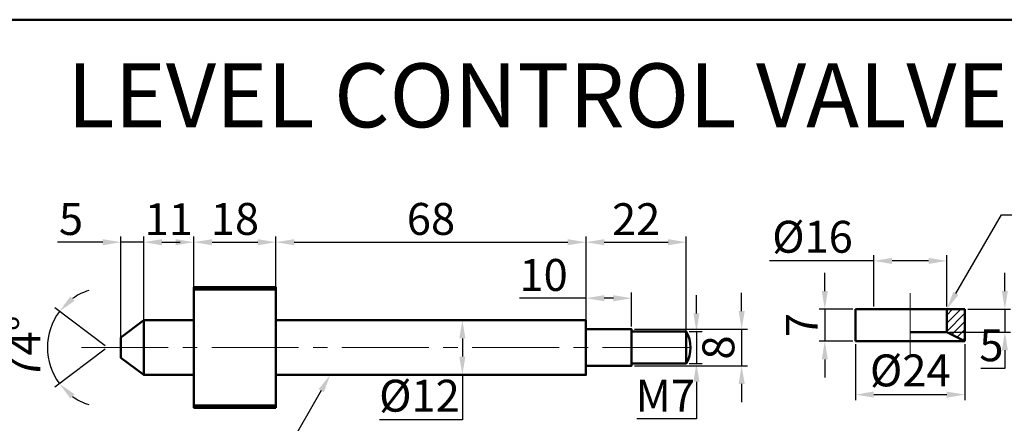
# Model space of a CAD drawing. Units: millimetres. Extents: x 123 to 731, y 468 to 864.
# Tile 4 of 5: x 328 to 544, y 775 to 864. Entities that reach past the tile are written whole.
import ezdxf
from ezdxf import colors
from ezdxf.entities.mleader import LeaderData, LeaderLine
from ezdxf.math import Vec2, Vec3

# ---------------------------------------------------------------- set-up
doc = ezdxf.new("R2010")
doc.units = ezdxf.units.MM
doc.linetypes.add('CENTER2', pattern=[28.575, 19.05, -3.175, 3.175, -3.175])
for name, color, linetype, lineweight in [('M-CNTR', 1, 'CENTER2', 18), ('M-DIMS', 2, 'Continuous', 25), ('M-HATC', 8, 'Continuous', 18), ('M-OUTL', 7, 'Continuous', 50), ('M-TEXT', 3, 'Continuous', 25)]:
    doc.layers.add(name, color=color, linetype=linetype, lineweight=lineweight)
doc.styles.get("Standard").update_dxf_attribs({"font": 'arial.ttf'})
doc.dimstyles.new('ISO-25', dxfattribs={"dimtxt": 7, "dimasz": 4, "dimexe": 1.25, "dimexo": 0.625, "dimtad": 1, "dimtoh": 1, "dimtxsty": 'Standard', "dimcen": 2.5, "dimadec": 0, "dimazin": 0, "dimtfac": 1, "dimtmove": 0, "dimatfit": 3, "dimfxl": 1, "dimarcsym": 0})

# ---------------------------------------------------------------- blocks, each defined once
blk = doc.blocks.new('*U27')
at = {"layer": 'M-CNTR', "color": 0, "transparency": 16777216}
blk.add_line((-76.67, 0), (58.73, 0), dxfattribs=at)
blk = doc.blocks.new('*D28')
at = {"layer": 'Defpoints', "color": 0, "transparency": 16777216}
for p in [(355.16, 798.03), (334.32, 794.85), (350.16, 794.26), (350.16, 789.8), (355.16, 786.03)]:
    blk.add_point(p, dxfattribs=at)
at = {"layer": 'M-DIMS', "color": 0, "lineweight": -2, "transparency": 16777216}
for p, q in [((346.7, 792.41), (335.67, 800.72)), ((346.7, 791.65), (335.67, 783.34))]:
    blk.add_line(p, q, dxfattribs=at)
for start, end in [(108.0972, 125.5486), (143, 217), (234.4514, 251.9028)]:
    blk.add_arc((347.2, 792.03), 13.18, start, end, dxfattribs=at)
at = {"layer": 'M-DIMS', "color": 0, "transparency": 16777216}
for points in [[(340, 802.28), (339.07, 803.23), (336.67, 799.97)], [(339.07, 780.83), (340, 781.78), (336.67, 784.1)]]:
    blk.add_solid(points, dxfattribs=at)
at = {"layer": 'M-DIMS', "color": 0, "transparency": 16777216, "insert": (329.89, 792.03), "char_height": 7, "attachment_point": 5, "rotation": 90}
blk.add_mtext('74°', dxfattribs=at)
blk = doc.blocks.new('*D29')
at = {"layer": 'Defpoints', "color": 0, "transparency": 16777216}
for p in [(355.16, 815.14), (350.16, 792.03), (355.16, 792.03)]:
    blk.add_point(p, dxfattribs=at)
at = {"layer": 'M-DIMS', "color": 0, "lineweight": -2, "transparency": 16777216}
for p, q in [((350.16, 792.66), (350.16, 816.39)), ((355.16, 792.66), (355.16, 816.39)), ((346.16, 815.14), (336.27, 815.14)), ((355.16, 815.14), (350.16, 815.14)), ((359.16, 815.14), (363.16, 815.14))]:
    blk.add_line(p, q, dxfattribs=at)
at = {"layer": 'M-DIMS', "color": 0, "transparency": 16777216}
for points in [[(346.16, 815.8), (346.16, 814.47), (350.16, 815.14)], [(359.16, 815.8), (359.16, 814.47), (355.16, 815.14)]]:
    blk.add_solid(points, dxfattribs=at)
at = {"layer": 'M-DIMS', "color": 0, "transparency": 16777216, "insert": (339.21, 819.32), "char_height": 7, "attachment_point": 5}
blk.add_mtext('5', dxfattribs=at)
blk = doc.blocks.new('*D30')
at = {"layer": 'Defpoints', "color": 0, "transparency": 16777216}
for p in [(366.16, 815.14), (355.16, 798.03), (366.16, 798.03)]:
    blk.add_point(p, dxfattribs=at)
at = {"layer": 'M-DIMS', "color": 0, "lineweight": -2, "transparency": 16777216}
for p, q in [((355.16, 798.66), (355.16, 816.39)), ((366.16, 798.66), (366.16, 816.39)), ((359.16, 815.14), (362.16, 815.14))]:
    blk.add_line(p, q, dxfattribs=at)
at = {"layer": 'M-DIMS', "color": 0, "transparency": 16777216}
for points in [[(359.16, 815.8), (359.16, 814.47), (355.16, 815.14)], [(362.16, 815.8), (362.16, 814.47), (366.16, 815.14)]]:
    blk.add_solid(points, dxfattribs=at)
at = {"layer": 'M-DIMS', "color": 0, "transparency": 16777216, "insert": (360.66, 819.28), "char_height": 7, "attachment_point": 5}
blk.add_mtext('11', dxfattribs=at)
blk = doc.blocks.new('*D31')
at = {"layer": 'Defpoints', "color": 0, "transparency": 16777216}
for p in [(384.16, 815.14), (366.16, 805.25), (384.16, 805.25)]:
    blk.add_point(p, dxfattribs=at)
at = {"layer": 'M-DIMS', "color": 0, "lineweight": -2, "transparency": 16777216}
for p, q in [((366.16, 805.88), (366.16, 816.39)), ((384.16, 805.88), (384.16, 816.39)), ((370.16, 815.14), (380.16, 815.14))]:
    blk.add_line(p, q, dxfattribs=at)
at = {"layer": 'M-DIMS', "color": 0, "transparency": 16777216}
for points in [[(370.16, 815.8), (370.16, 814.47), (366.16, 815.14)], [(380.16, 815.8), (380.16, 814.47), (384.16, 815.14)]]:
    blk.add_solid(points, dxfattribs=at)
at = {"layer": 'M-DIMS', "color": 0, "transparency": 16777216, "insert": (375.16, 819.34), "char_height": 7, "attachment_point": 5}
blk.add_mtext('18', dxfattribs=at)
blk = doc.blocks.new('*D32')
at = {"layer": 'Defpoints', "color": 0, "transparency": 16777216}
for p in [(452.16, 815.14), (384.16, 798.03), (452.16, 796.03)]:
    blk.add_point(p, dxfattribs=at)
at = {"layer": 'M-DIMS', "color": 0, "lineweight": -2, "transparency": 16777216}
for p, q in [((384.16, 798.66), (384.16, 816.39)), ((452.16, 796.66), (452.16, 816.39)), ((388.16, 815.14), (448.16, 815.14))]:
    blk.add_line(p, q, dxfattribs=at)
at = {"layer": 'M-DIMS', "color": 0, "transparency": 16777216}
for points in [[(388.16, 815.8), (388.16, 814.47), (384.16, 815.14)], [(448.16, 815.8), (448.16, 814.47), (452.16, 815.14)]]:
    blk.add_solid(points, dxfattribs=at)
at = {"layer": 'M-DIMS', "color": 0, "transparency": 16777216, "insert": (418.16, 819.34), "char_height": 7, "attachment_point": 5}
blk.add_mtext('68', dxfattribs=at)
blk = doc.blocks.new('*D33')
at = {"layer": 'Defpoints', "color": 0, "transparency": 16777216}
for p in [(474.16, 815.14), (452.16, 796.03), (474.16, 792.03)]:
    blk.add_point(p, dxfattribs=at)
at = {"layer": 'M-DIMS', "color": 0, "lineweight": -2, "transparency": 16777216}
for p, q in [((452.16, 796.66), (452.16, 816.39)), ((474.16, 792.66), (474.16, 816.39)), ((456.16, 815.14), (470.16, 815.14))]:
    blk.add_line(p, q, dxfattribs=at)
at = {"layer": 'M-DIMS', "color": 0, "transparency": 16777216}
for points in [[(456.16, 815.8), (456.16, 814.47), (452.16, 815.14)], [(470.16, 815.8), (470.16, 814.47), (474.16, 815.14)]]:
    blk.add_solid(points, dxfattribs=at)
at = {"layer": 'M-DIMS', "color": 0, "transparency": 16777216, "insert": (463.16, 819.28), "char_height": 7, "attachment_point": 5}
blk.add_mtext('22', dxfattribs=at)
blk = doc.blocks.new('*D34')
at = {"layer": 'Defpoints', "color": 0, "transparency": 16777216}
for p in [(425.65, 798.03), (425.04, 786.03), (425.65, 786.03)]:
    blk.add_point(p, dxfattribs=at)
at = {"layer": 'M-DIMS', "color": 0, "lineweight": -2, "transparency": 16777216}
for p, q in [((425.03, 798.03), (423.79, 798.03)), ((425.04, 794.03), (425.04, 790.03)), ((425.03, 786.03), (423.79, 786.03)), ((425.04, 786.03), (425.04, 776.16)), ((425.04, 776.16), (406.85, 776.16))]:
    blk.add_line(p, q, dxfattribs=at)
at = {"layer": 'M-DIMS', "color": 0, "transparency": 16777216}
for points in [[(424.38, 794.03), (425.71, 794.03), (425.04, 798.03)], [(424.38, 790.03), (425.71, 790.03), (425.04, 786.03)]]:
    blk.add_solid(points, dxfattribs=at)
at = {"layer": 'M-DIMS', "color": 0, "transparency": 16777216, "insert": (415.63, 780.55), "char_height": 7, "attachment_point": 5}
blk.add_mtext('%%C12', dxfattribs=at)
blk = doc.blocks.new('*D35')
at = {"layer": 'Defpoints', "color": 0, "transparency": 16777216}
for p in [(462.16, 802.85), (452.16, 796.03), (462.16, 796.03)]:
    blk.add_point(p, dxfattribs=at)
at = {"layer": 'M-DIMS', "color": 0, "lineweight": -2, "transparency": 16777216}
for p, q in [((452.16, 796.66), (452.16, 804.1)), ((462.16, 796.66), (462.16, 804.1)), ((452.16, 802.85), (437.56, 802.85)), ((458.16, 802.85), (456.16, 802.85))]:
    blk.add_line(p, q, dxfattribs=at)
at = {"layer": 'M-DIMS', "color": 0, "transparency": 16777216}
for points in [[(456.16, 803.51), (456.16, 802.18), (452.16, 802.85)], [(458.16, 803.51), (458.16, 802.18), (462.16, 802.85)]]:
    blk.add_solid(points, dxfattribs=at)
at = {"layer": 'M-DIMS', "color": 0, "transparency": 16777216, "insert": (442.86, 807.05), "char_height": 7, "attachment_point": 5}
blk.add_mtext('10', dxfattribs=at)
blk = doc.blocks.new('*D36')
at = {"layer": 'Defpoints', "color": 0, "transparency": 16777216}
for p in [(474.16, 795.53), (474.16, 788.53), (476.38, 788.53)]:
    blk.add_point(p, dxfattribs=at)
at = {"layer": 'M-DIMS', "color": 0, "lineweight": -2, "transparency": 16777216}
for p, q in [((476.38, 799.53), (476.38, 803.53)), ((474.78, 795.53), (477.63, 795.53)), ((476.38, 795.53), (476.38, 788.53)), ((474.78, 788.53), (477.63, 788.53)), ((476.38, 784.53), (476.38, 776.41)), ((476.38, 776.41), (463.34, 776.41))]:
    blk.add_line(p, q, dxfattribs=at)
at = {"layer": 'M-DIMS', "color": 0, "transparency": 16777216}
for points in [[(475.72, 799.53), (477.05, 799.53), (476.38, 795.53)], [(475.72, 784.53), (477.05, 784.53), (476.38, 788.53)]]:
    blk.add_solid(points, dxfattribs=at)
at = {"layer": 'M-DIMS', "color": 0, "transparency": 16777216, "insert": (469.55, 780.54), "char_height": 7, "attachment_point": 5}
blk.add_mtext('M7', dxfattribs=at)
blk = doc.blocks.new('*D37')
at = {"layer": 'Defpoints', "color": 0, "transparency": 16777216}
for p in [(462.16, 796.03), (462.16, 788.03), (486.3, 788.03)]:
    blk.add_point(p, dxfattribs=at)
at = {"layer": 'M-DIMS', "color": 0, "lineweight": -2, "transparency": 16777216}
for p, q in [((486.3, 800.03), (486.3, 804.03)), ((462.78, 796.03), (487.55, 796.03)), ((486.3, 796.03), (486.3, 788.03)), ((462.78, 788.03), (487.55, 788.03)), ((486.3, 784.03), (486.3, 780.03))]:
    blk.add_line(p, q, dxfattribs=at)
at = {"layer": 'M-DIMS', "color": 0, "transparency": 16777216}
for points in [[(485.63, 800.03), (486.97, 800.03), (486.3, 796.03)], [(485.63, 784.03), (486.97, 784.03), (486.3, 788.03)]]:
    blk.add_solid(points, dxfattribs=at)
at = {"layer": 'M-DIMS', "color": 0, "transparency": 16777216, "insert": (482.1, 792.03), "char_height": 7, "attachment_point": 5, "rotation": 90}
blk.add_mtext('8', dxfattribs=at)
blk = doc.blocks.new('*U49')
at = {"layer": 'M-CNTR', "color": 0, "transparency": 16777216}
blk.add_line((0, 7), (0, -7), dxfattribs=at)
blk = doc.blocks.new('*D50')
at = {"layer": 'Defpoints', "color": 0, "transparency": 16777216}
for p in [(511.28, 793.43), (535.28, 793.43), (535.28, 781.7)]:
    blk.add_point(p, dxfattribs=at)
at = {"layer": 'M-DIMS', "color": 0, "lineweight": -2, "transparency": 16777216}
for p, q in [((511.28, 792.8), (511.28, 780.45)), ((535.28, 792.8), (535.28, 780.45)), ((515.28, 781.7), (531.28, 781.7))]:
    blk.add_line(p, q, dxfattribs=at)
at = {"layer": 'M-DIMS', "color": 0, "transparency": 16777216}
for points in [[(515.28, 782.37), (515.28, 781.03), (511.28, 781.7)], [(531.28, 782.37), (531.28, 781.03), (535.28, 781.7)]]:
    blk.add_solid(points, dxfattribs=at)
at = {"layer": 'M-DIMS', "color": 0, "transparency": 16777216, "insert": (523.28, 786.1), "char_height": 7, "attachment_point": 5}
blk.add_mtext('%%C24', dxfattribs=at)
blk = doc.blocks.new('*D51')
at = {"layer": 'Defpoints', "color": 0, "transparency": 16777216}
for p in [(535.28, 800.43), (531.28, 795.43), (544.03, 795.43)]:
    blk.add_point(p, dxfattribs=at)
at = {"layer": 'M-DIMS', "color": 0, "lineweight": -2, "transparency": 16777216}
for p, q in [((544.03, 804.43), (544.03, 808.43)), ((535.9, 800.43), (545.28, 800.43)), ((544.03, 800.43), (544.03, 795.43)), ((531.9, 795.43), (545.28, 795.43)), ((544.03, 791.43), (544.03, 787.43)), ((544.03, 787.43), (538.76, 787.43))]:
    blk.add_line(p, q, dxfattribs=at)
at = {"layer": 'M-DIMS', "color": 0, "transparency": 16777216}
for points in [[(543.36, 804.43), (544.69, 804.43), (544.03, 800.43)], [(543.36, 791.43), (544.69, 791.43), (544.03, 795.43)]]:
    blk.add_solid(points, dxfattribs=at)
at = {"layer": 'M-DIMS', "color": 0, "transparency": 16777216, "insert": (541.08, 791.61), "char_height": 7, "attachment_point": 5}
blk.add_mtext('5', dxfattribs=at)
blk = doc.blocks.new('*D52')
at = {"layer": 'Defpoints', "color": 0, "transparency": 16777216}
for p in [(511.28, 800.43), (504.53, 793.43), (511.28, 793.43)]:
    blk.add_point(p, dxfattribs=at)
at = {"layer": 'M-DIMS', "color": 0, "lineweight": -2, "transparency": 16777216}
for p, q in [((504.53, 804.43), (504.53, 808.43)), ((510.65, 800.43), (503.28, 800.43)), ((504.53, 800.43), (504.53, 793.43)), ((510.65, 793.43), (503.28, 793.43)), ((504.53, 789.43), (504.53, 785.43))]:
    blk.add_line(p, q, dxfattribs=at)
at = {"layer": 'M-DIMS', "color": 0, "transparency": 16777216}
for points in [[(503.87, 804.43), (505.2, 804.43), (504.53, 800.43)], [(503.87, 789.43), (505.2, 789.43), (504.53, 793.43)]]:
    blk.add_solid(points, dxfattribs=at)
at = {"layer": 'M-DIMS', "color": 0, "transparency": 16777216, "insert": (500.41, 796.93), "char_height": 7, "attachment_point": 5, "rotation": 90}
blk.add_mtext('7', dxfattribs=at)
blk = doc.blocks.new('*D53')
at = {"layer": 'Defpoints', "color": 0, "transparency": 16777216}
for p in [(515.28, 811.03), (515.28, 800.43), (531.28, 800.43)]:
    blk.add_point(p, dxfattribs=at)
at = {"layer": 'M-DIMS', "color": 0, "lineweight": -2, "transparency": 16777216}
for p, q in [((515.28, 801.05), (515.28, 812.28)), ((531.28, 801.05), (531.28, 812.28)), ((515.28, 811.03), (492.39, 811.03)), ((527.28, 811.03), (519.28, 811.03))]:
    blk.add_line(p, q, dxfattribs=at)
at = {"layer": 'M-DIMS', "color": 0, "transparency": 16777216}
for points in [[(519.28, 811.7), (519.28, 810.36), (515.28, 811.03)], [(527.28, 811.7), (527.28, 810.36), (531.28, 811.03)]]:
    blk.add_solid(points, dxfattribs=at)
at = {"layer": 'M-DIMS', "color": 0, "transparency": 16777216, "insert": (501.84, 815.42), "char_height": 7, "attachment_point": 5}
blk.add_mtext('%%C16', dxfattribs=at)

msp = doc.modelspace()

# ---------------------------------------------------------------- hatches: boundary and pattern name
at = {"layer": 'M-HATC'}
h = msp.add_hatch(dxfattribs=at)
h.set_pattern_fill('ANSI31', color=256, scale=0.4)
h.set_pattern_definition([(45, (-4.0036, 30.3746), (-0.8980256, 0.8980256), [])])
h.paths.add_polyline_path([(535.2797, 800.4278), (531.2797, 800.4278), (531.2797, 795.4278), (535.2797, 793.4278)])

# ---------------------------------------------------------------- linework, layer by layer
at = {"layer": 'M-OUTL'}
for p, q in [((384.1582, 804.7511), (366.1582, 804.7511)), ((535.2797, 800.4278), (511.2797, 800.4278)), ((511.2797, 800.4278), (511.2797, 793.4278)), ((531.2797, 800.4278), (531.2797, 795.4278)), ((535.2797, 793.4278), (535.2797, 800.4278)), ((366.1582, 798.0311), (355.1582, 798.0311)), ((531.2797, 795.4278), (523.2797, 795.4278)), ((531.2797, 795.4278), (535.2797, 793.4278)), ((511.2797, 793.4278), (535.2797, 793.4278)), ((366.1582, 779.3111), (384.1582, 779.3111))]:
    msp.add_line(p, q, dxfattribs=at)
for points in [[(123.3719, 863.9604), (731.4761, 863.9604), (731.4761, 468.4518), (123.3719, 468.4518)], [(384.1582, 778.8111), (384.1582, 805.2511), (366.1582, 805.2511), (366.1582, 778.8111)]]:
    msp.add_lwpolyline(points, close=True, dxfattribs=at)
for points in [[(355.1582, 786.0311), (355.1582, 798.0311), (350.1582, 794.2634), (350.1582, 789.7989), (355.1582, 786.0311), (366.1582, 786.0311)], [(384.1582, 798.0311), (452.1582, 798.0311), (452.1582, 786.0311), (384.1582, 786.0311)], [(452.1582, 796.0311), (462.1582, 796.0311), (462.1582, 788.0311), (452.1582, 788.0311)], [(462.1582, 795.5311), (474.1582, 795.5311), (474.1582, 788.5311), (462.1582, 788.5311)]]:
    msp.add_lwpolyline(points, dxfattribs=at)
msp.add_arc((468.096, 792.0311), 7, 330, 30, dxfattribs=at)

# ---------------------------------------------------------------- block references
at = {"layer": 'M-CNTR'}
for name, p in [('*U49', (523.2797, 796.9278)), ('*U27', (418.1582, 792.0311))]:
    msp.add_blockref(name, p, dxfattribs=at)

# ---------------------------------------------------------------- texts
at = {"layer": 'M-TEXT', "insert": (338.3996, 854.3546), "char_height": 14, "attachment_point": 1}
msp.add_mtext_dynamic_manual_height_columns('LEVEL CONTROL VALVE', width=267.64526, gutter_width=12.5, heights=[0], dxfattribs=at)

# ---------------------------------------------------------------- dimensions: what is measured, and where the dimension line sits
at = {"layer": 'M-DIMS'}
for base, p1, p2, picture, middle in [((355.1582, 815.1363), (350.1582, 792.0311), (355.1582, 792.0311), '*D29', (339.2126, 815.1363)), ((462.1582, 802.8462), (452.1582, 796.0311), (462.1582, 796.0311), '*D35', (442.861, 802.8462))]:
    dim = msp.add_linear_dim(base=base, p1=p1, p2=p2, dimstyle='ISO-25', override={"dimclrd": 0, "dimclre": 0, "dimclrt": 0}, dxfattribs=at)
    dim.commit()
    dim.dimension.update_dxf_attribs({"geometry": picture, "text_midpoint": middle, "dimtype": 160})
for base, p1, p2, picture, middle in [((366.1582, 815.1363), (355.1582, 798.0311), (366.1582, 798.0311), '*D30', (360.6582, 819.2756)), ((384.1582, 815.1363), (366.1582, 805.2511), (384.1582, 805.2511), '*D31', (375.1582, 819.3353)), ((452.1582, 815.1363), (384.1582, 798.0311), (452.1582, 796.0311), '*D32', (418.1582, 819.3353)), ((474.1582, 815.1363), (452.1582, 796.0311), (474.1582, 792.0311), '*D33', (463.1582, 819.2756))]:
    dim = msp.add_linear_dim(base=base, p1=p1, p2=p2, dimstyle='ISO-25', override={"dimclrd": 0, "dimclre": 0, "dimclrt": 0}, dxfattribs=at)
    dim.commit()
    dim.dimension.update_dxf_attribs({"geometry": picture, "text_midpoint": middle})
dim = msp.add_linear_dim(base=(515.2797, 811.03), p1=(531.2797, 800.4278), p2=(515.2797, 800.4278), text='%%C<>', dimstyle='ISO-25', override={"dimclrd": 0, "dimclre": 0, "dimclrt": 0}, dxfattribs=at)
dim.commit()
dim.dimension.update_dxf_attribs({"geometry": '*D53', "text_midpoint": (501.8355, 811.03), "dimtype": 160})
for base, p1, p2, picture, middle in [((504.5338, 793.4278), (511.2797, 800.4278), (511.2797, 793.4278), '*D52', (500.4088, 796.9278)), ((544.027, 795.4278), (535.2797, 800.4278), (531.2797, 795.4278), '*D51', (541.0814, 791.6125)), ((486.3013, 788.0311), (462.1582, 796.0311), (462.1582, 788.0311), '*D37', (482.1023, 792.0311))]:
    dim = msp.add_linear_dim(base=base, p1=p1, p2=p2, angle=90, dimstyle='ISO-25', override={"dimclrd": 0, "dimclre": 0, "dimclrt": 0}, dxfattribs=at)
    dim.commit()
    dim.dimension.update_dxf_attribs({"geometry": picture, "text_midpoint": middle})
dim = msp.add_angular_dim_2l(base=(334.3166, 794.8471), line1=((350.1582, 789.7989), (355.1582, 786.0311)), line2=((355.1582, 798.0311), (350.1582, 794.2634)), dimstyle='ISO-25', override={"dimclrd": 0, "dimclre": 0, "dimclrt": 0}, dxfattribs=at)
dim.commit()
dim.dimension.update_dxf_attribs({"geometry": '*D28', "text_midpoint": (329.8874, 792.0311)})
for base, p1, p2, text, picture, middle in [((476.3843, 788.5311), (474.1582, 795.5311), (474.1582, 788.5311), 'M<>', '*D36', (469.5519, 776.4148)), ((425.044, 786.0311), (425.6508, 798.0311), (425.6508, 786.0311), '%%C<>', '*D34', (415.6332, 776.1585))]:
    dim = msp.add_linear_dim(base=base, p1=p1, p2=p2, angle=90, text=text, dimstyle='ISO-25', override={"dimclrd": 0, "dimclre": 0, "dimclrt": 0}, dxfattribs=at)
    dim.commit()
    dim.dimension.update_dxf_attribs({"geometry": picture, "text_midpoint": middle, "dimtype": 160})
dim = msp.add_linear_dim(base=(535.2797, 781.7007), p1=(511.2797, 793.4278), p2=(535.2797, 793.4278), text='%%C<>', dimstyle='ISO-25', override={"dimclrd": 0, "dimclre": 0, "dimclrt": 0}, dxfattribs=at)
dim.commit()
dim.dimension.update_dxf_attribs({"geometry": '*D50', "text_midpoint": (523.2797, 786.0955)})

# ---------------------------------------------------------------- leaders
at = {"layer": 'M-TEXT'}
ml = msp.add_multileader_mtext('Standard', dxfattribs=at)
ml.set_content('12', color=256)
ml.set_leader_properties()
ml.build(insert=Vec2(0, 0))
ctx = ml.context
ctx.base_point, ctx.char_height, ctx.plane_origin = Vec3(551.2554, 821.1704), 15, Vec3(531.2797, 800.4278)
notes = []
notes.append((ctx, [(0, (1, 1, 0), (543.2554, 821.1704), (1, 0), 8, [(0, [(531.2797, 800.4278)], 0, [])])]))
ctx.mtext.insert, ctx.mtext.flow_direction = Vec3(553.2554, 828.6704), 5
ml = msp.add_multileader_mtext('Standard', dxfattribs=at)
ml.set_content('9', color=256)
ml.set_leader_properties()
ml.build(insert=Vec2(0, 0))
ctx = ml.context
ctx.base_point, ctx.char_height, ctx.plane_origin = Vec3(361.9336, 764.7505), 15, Vec3(396.0835, 786.0311)
ctx.text_align_type = 2
notes.append((ctx, [(0, (1, 1, 0), (383.7971, 764.7505), (-1, 0), 8, [(0, [(396.0835, 786.0311)], 0, [])])]))
ctx.mtext.insert, ctx.mtext.alignment, ctx.mtext.flow_direction = Vec3(373.7971, 772.3784), 3, 5
for ctx, leaders in notes:
    for number, flags, end, landing, length, lines in leaders:
        leader = LeaderData()
        leader.index, (leader.has_last_leader_line, leader.has_dogleg_vector, leader.attachment_direction) = number, flags
        leader.last_leader_point, leader.dogleg_vector, leader.dogleg_length = Vec3(end), Vec3(landing), length
        for number, points, colour, breaks in lines:
            line = LeaderLine()
            line.index, line.vertices, line.color, line.breaks = number, Vec3.list(points), colors.encode_raw_color(colour), breaks
            leader.lines.append(line)
        ctx.leaders.append(leader)

doc.saveas('drawing.dxf')
